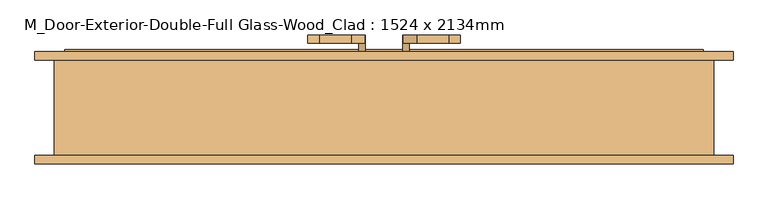
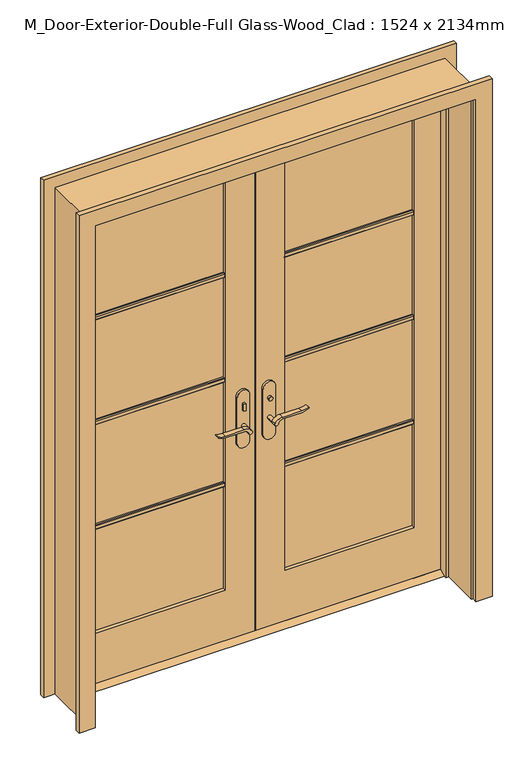
"""IFC4 building model written with IfcOpenShell, lengths in millimetres: door geometry, M_Door-Exterior-Double-Full Glass-Wood_Clad : 1524 x 2134mm."""

from ifc_helpers import new_model, si_unit, point, frame, frame_2d, origin, place, context, project, spatial, polyline, circle_curve, trimmed, segment, composite_curve, outline, extrude, faceted_brep, source, transform, mapped, element, save


def m_door_exterior_double_full_glass_wood_clad_1524_x_2134mm_606f56d5(model_context):
    return source(origin(), model_context, "Body", "SolidModel", [
        extrude(outline(polyline([(76.125, 15.0), (111.125, 15.0), (136.525, 0.0), (50.725, 0.0), (76.125, 15.0)])), frame((-762.0, 0.0, 0.0), z_axis=(1.0, 0.0, 0.0), x_axis=(0.0, 1.0, 0.0)), (0.0, 0.0, 1.0), 1524.0),
        extrude(outline(polyline([(-47.4019111, 56.125), (-57.4019111, 56.125), (-57.4019111, 66.125), (-47.4019111, 66.125), (-47.4019111, 56.125)])), frame((0.0, 0.0, 981.9), z_axis=(0.0, 0.0, 1.0), x_axis=(1.0, 0.0, 0.0)), (0.0, 0.0, 1.0), 30.0),
        extrude(outline(composite_curve([segment(trimmed(circle_curve(frame_2d((996.9, -52.4019111)), 8.0), [point((996.9, -60.4019111))], [point((996.9, -44.4019111))], False, "CARTESIAN"), True, "CONTINUOUS"), segment(trimmed(circle_curve(frame_2d((996.9, -52.4019111)), 8.0), [point((996.9, -44.4019111))], [point((996.9, -60.4019111))], False, "CARTESIAN"), True, "CONTINUOUS")], self_intersect=False)), frame((0.0, 121.125, 0.0), z_axis=(0.0, 1.0, 0.0), x_axis=(0.0, 0.0, 1.0)), (0.0, 0.0, 1.0), 10.0),
        extrude(outline(composite_curve([segment(trimmed(circle_curve(frame_2d((897.1555521, -76.0694241)), 37.2832219), [point((919.0523287, -45.8937749))], [point((934.4, -77.7693445))], False, "CARTESIAN"), True, "CONTINUOUS"), segment(polyline([(934.4, -77.7693445), (934.4, -154.045502)]), True, "CONTINUOUS"), segment(trimmed(circle_curve(frame_2d((1017.6850638, -153.9791202)), 83.2850902), [point((934.4, -154.045502))], [point((939.4, -182.4019111))], True, "CARTESIAN"), True, "CONTINUOUS"), segment(polyline([(939.4, -182.4019111), (936.6135558, -182.4019111)]), True, "CONTINUOUS"), segment(trimmed(circle_curve(frame_2d((986.6709207, -150.4622499)), 59.3791355), [point((936.6135558, -182.4019111))], [point((927.4, -154.045502))], False, "CARTESIAN"), True, "CONTINUOUS"), segment(polyline([(927.4, -154.045502), (927.4, -77.7881013)]), True, "CONTINUOUS"), segment(trimmed(circle_curve(frame_2d((909.2738613, -77.7881013)), 18.1261387), [point((927.4, -77.7881013))], [point((914.4, -60.4019111))], True, "CARTESIAN"), True, "CONTINUOUS"), segment(trimmed(circle_curve(frame_2d((914.4, -52.4019111)), 8.0), [point((914.4, -60.4019111))], [point((919.0523287, -45.8937749))], False, "CARTESIAN"), True, "CONTINUOUS")], self_intersect=False)), frame((0.0, 16.125, 0.0), z_axis=(0.0, 1.0, 0.0), x_axis=(0.0, 0.0, 1.0)), (0.0, 0.0, 1.0), 20.0),
        extrude(outline(composite_curve([segment(trimmed(circle_curve(frame_2d((914.4, -52.4019111)), 8.0), [point((914.3999903, -60.4019111))], [point((919.0523287, -45.8937749))], False, "CARTESIAN"), True, "CONTINUOUS"), segment(trimmed(circle_curve(frame_2d((897.1555521, -76.0694241)), 37.2832219), [point((919.0523287, -45.8937749))], [point((934.4, -77.7693445))], False, "CARTESIAN"), True, "CONTINUOUS"), segment(polyline([(934.4, -77.7693445), (934.4, -154.045502)]), True, "CONTINUOUS"), segment(trimmed(circle_curve(frame_2d((1017.6850638, -153.9791202)), 83.2850902), [point((934.4, -154.045502))], [point((939.4, -182.4019111))], True, "CARTESIAN"), True, "CONTINUOUS"), segment(polyline([(939.4, -182.4019111), (936.6135558, -182.4019111)]), True, "CONTINUOUS"), segment(trimmed(circle_curve(frame_2d((986.6709207, -150.4622499)), 59.3791355), [point((936.6135558, -182.4019111))], [point((927.4, -154.045502))], False, "CARTESIAN"), True, "CONTINUOUS"), segment(polyline([(927.4, -154.045502), (927.4, -77.788099)]), True, "CONTINUOUS"), segment(trimmed(circle_curve(frame_2d((909.2738682, -77.788099)), 18.1261318), [point((927.4, -77.788099))], [point((914.3999903, -60.4019111))], True, "CARTESIAN"), True, "CONTINUOUS")], self_intersect=False)), frame((0.0, 151.125, 0.0), z_axis=(0.0, 1.0, 0.0), x_axis=(0.0, 0.0, 1.0)), (0.0, 0.0, 1.0), 20.0),
        extrude(outline(composite_curve([segment(trimmed(circle_curve(frame_2d((914.4, -52.4019111)), 8.0), [point((914.4, -60.4019111))], [point((914.4, -44.4019111))], False, "CARTESIAN"), True, "CONTINUOUS"), segment(trimmed(circle_curve(frame_2d((914.4, -52.4019111)), 8.0), [point((914.4, -44.4019111))], [point((914.4, -60.4019111))], False, "CARTESIAN"), True, "CONTINUOUS")], self_intersect=False)), frame((0.0, 36.125, 0.0), z_axis=(0.0, 1.0, 0.0), x_axis=(0.0, 0.0, 1.0)), (0.0, 0.0, 1.0), 30.0),
        extrude(outline(composite_curve([segment(trimmed(circle_curve(frame_2d((914.4, -52.4019111)), 8.0), [point((914.4, -60.4019111))], [point((914.4, -44.4019111))], False, "CARTESIAN"), True, "CONTINUOUS"), segment(trimmed(circle_curve(frame_2d((914.4, -52.4019111)), 8.0), [point((914.4, -44.4019111))], [point((914.4, -60.4019111))], False, "CARTESIAN"), True, "CONTINUOUS")], self_intersect=False)), frame((0.0, 121.125, 0.0), z_axis=(0.0, 1.0, 0.0), x_axis=(0.0, 0.0, 1.0)), (0.0, 0.0, 1.0), 30.0),
        extrude(outline(composite_curve([segment(polyline([(844.4, -27.4019111), (1039.4, -27.4019111)]), True, "CONTINUOUS"), segment(trimmed(circle_curve(frame_2d((1039.4, -52.4019111)), 25.0), [point((1039.4, -27.4019111))], [point((1039.4, -77.4019111))], False, "CARTESIAN"), True, "CONTINUOUS"), segment(polyline([(1039.4, -77.4019111), (844.4, -77.4019111)]), True, "CONTINUOUS"), segment(trimmed(circle_curve(frame_2d((844.4, -52.4019111)), 25.0), [point((844.4, -77.4019111))], [point((844.4, -27.4019111))], False, "CARTESIAN"), True, "CONTINUOUS")], self_intersect=False)), frame((0.0, 66.125, 0.0), z_axis=(0.0, 1.0, 0.0), x_axis=(0.0, 0.0, 1.0)), (0.0, 0.0, 1.0), 10.0),
        extrude(outline(composite_curve([segment(polyline([(844.4, -27.4019111), (1039.4, -27.4019111)]), True, "CONTINUOUS"), segment(trimmed(circle_curve(frame_2d((1039.4, -52.4019111)), 25.0), [point((1039.4, -27.4019111))], [point((1039.4, -77.4019111))], False, "CARTESIAN"), True, "CONTINUOUS"), segment(polyline([(1039.4, -77.4019111), (844.4, -77.4019111)]), True, "CONTINUOUS"), segment(trimmed(circle_curve(frame_2d((844.4, -52.4019111)), 25.0), [point((844.4, -77.4019111))], [point((844.4, -27.4019111))], False, "CARTESIAN"), True, "CONTINUOUS")], self_intersect=False)), frame((0.0, 111.125, 0.0), z_axis=(0.0, 1.0, 0.0), x_axis=(0.0, 0.0, 1.0)), (0.0, 0.0, 1.0), 10.0),
        extrude(outline(polyline([(47.3875, 131.125), (57.3875, 131.125), (57.3875, 121.125), (47.3875, 121.125), (47.3875, 131.125)])), frame((0.0, 0.0, 981.9), z_axis=(0.0, 0.0, 1.0), x_axis=(1.0, 0.0, 0.0)), (0.0, 0.0, 1.0), 30.0),
        extrude(outline(composite_curve([segment(trimmed(circle_curve(frame_2d((996.9, 52.3875)), 8.0), [point((996.9, 60.3875))], [point((996.9, 44.3875))], False, "CARTESIAN"), True, "CONTINUOUS"), segment(trimmed(circle_curve(frame_2d((996.9, 52.3875)), 8.0), [point((996.9, 44.3875))], [point((996.9, 60.3875))], False, "CARTESIAN"), True, "CONTINUOUS")], self_intersect=False)), frame((0.0, 56.125, 0.0), z_axis=(0.0, 1.0, 0.0), x_axis=(0.0, 0.0, 1.0)), (0.0, 0.0, 1.0), 10.0),
        extrude(outline(composite_curve([segment(trimmed(circle_curve(frame_2d((914.4, 52.3875)), 8.0), [point((919.0523287, 45.8793637))], [point((914.4, 60.3875))], False, "CARTESIAN"), True, "CONTINUOUS"), segment(trimmed(circle_curve(frame_2d((909.2738613, 77.7736901)), 18.1261387), [point((914.4, 60.3875))], [point((927.4, 77.7736901))], True, "CARTESIAN"), True, "CONTINUOUS"), segment(polyline([(927.4, 77.7736901), (927.4, 154.0310909)]), True, "CONTINUOUS"), segment(trimmed(circle_curve(frame_2d((986.6709207, 150.4478388)), 59.3791355), [point((927.4, 154.0310909))], [point((936.6135558, 182.3875))], False, "CARTESIAN"), True, "CONTINUOUS"), segment(polyline([(936.6135558, 182.3875), (939.4, 182.3875)]), True, "CONTINUOUS"), segment(trimmed(circle_curve(frame_2d((1017.6850638, 153.9647091)), 83.2850902), [point((939.4, 182.3875))], [point((934.4, 154.0310909))], True, "CARTESIAN"), True, "CONTINUOUS"), segment(polyline([(934.4, 154.0310909), (934.4, 77.7549333)]), True, "CONTINUOUS"), segment(trimmed(circle_curve(frame_2d((897.1555521, 76.0550129)), 37.2832219), [point((934.4, 77.7549333))], [point((919.0523287, 45.8793637))], False, "CARTESIAN"), True, "CONTINUOUS")], self_intersect=False)), frame((0.0, 151.125, 0.0), z_axis=(0.0, 1.0, 0.0), x_axis=(0.0, 0.0, 1.0)), (0.0, 0.0, 1.0), 20.0),
        extrude(outline(composite_curve([segment(trimmed(circle_curve(frame_2d((909.2738682, 77.7736878)), 18.1261318), [point((914.3999903, 60.3875))], [point((927.4, 77.7736878))], True, "CARTESIAN"), True, "CONTINUOUS"), segment(polyline([(927.4, 77.7736878), (927.4, 154.0310909)]), True, "CONTINUOUS"), segment(trimmed(circle_curve(frame_2d((986.6709207, 150.4478388)), 59.3791355), [point((927.4, 154.0310909))], [point((936.6135558, 182.3875))], False, "CARTESIAN"), True, "CONTINUOUS"), segment(polyline([(936.6135558, 182.3875), (939.4, 182.3875)]), True, "CONTINUOUS"), segment(trimmed(circle_curve(frame_2d((1017.6850638, 153.9647091)), 83.2850902), [point((939.4, 182.3875))], [point((934.4, 154.0310909))], True, "CARTESIAN"), True, "CONTINUOUS"), segment(polyline([(934.4, 154.0310909), (934.4, 77.7549333)]), True, "CONTINUOUS"), segment(trimmed(circle_curve(frame_2d((897.1555521, 76.0550129)), 37.2832219), [point((934.4, 77.7549333))], [point((919.0523287, 45.8793637))], False, "CARTESIAN"), True, "CONTINUOUS"), segment(trimmed(circle_curve(frame_2d((914.4, 52.3875)), 8.0), [point((919.0523287, 45.8793637))], [point((914.3999903, 60.3875))], False, "CARTESIAN"), True, "CONTINUOUS")], self_intersect=False)), frame((0.0, 16.125, 0.0), z_axis=(0.0, 1.0, 0.0), x_axis=(0.0, 0.0, 1.0)), (0.0, 0.0, 1.0), 20.0),
        extrude(outline(composite_curve([segment(trimmed(circle_curve(frame_2d((914.4, 52.3875)), 8.0), [point((914.4, 60.3875))], [point((914.4, 44.3875))], False, "CARTESIAN"), True, "CONTINUOUS"), segment(trimmed(circle_curve(frame_2d((914.4, 52.3875)), 8.0), [point((914.4, 44.3875))], [point((914.4, 60.3875))], False, "CARTESIAN"), True, "CONTINUOUS")], self_intersect=False)), frame((0.0, 121.125, 0.0), z_axis=(0.0, 1.0, 0.0), x_axis=(0.0, 0.0, 1.0)), (0.0, 0.0, 1.0), 30.0),
        extrude(outline(composite_curve([segment(trimmed(circle_curve(frame_2d((914.4, 52.3875)), 8.0), [point((914.4, 60.3875))], [point((914.4, 44.3875))], False, "CARTESIAN"), True, "CONTINUOUS"), segment(trimmed(circle_curve(frame_2d((914.4, 52.3875)), 8.0), [point((914.4, 44.3875))], [point((914.4, 60.3875))], False, "CARTESIAN"), True, "CONTINUOUS")], self_intersect=False)), frame((0.0, 36.125, 0.0), z_axis=(0.0, 1.0, 0.0), x_axis=(0.0, 0.0, 1.0)), (0.0, 0.0, 1.0), 30.0),
        extrude(outline(composite_curve([segment(trimmed(circle_curve(frame_2d((844.4, 52.3875)), 25.0), [point((844.4, 27.3875))], [point((844.4, 77.3875))], False, "CARTESIAN"), True, "CONTINUOUS"), segment(polyline([(844.4, 77.3875), (1039.4, 77.3875)]), True, "CONTINUOUS"), segment(trimmed(circle_curve(frame_2d((1039.4, 52.3875)), 25.0), [point((1039.4, 77.3875))], [point((1039.4, 27.3875))], False, "CARTESIAN"), True, "CONTINUOUS"), segment(polyline([(1039.4, 27.3875), (844.4, 27.3875)]), True, "CONTINUOUS")], self_intersect=False)), frame((0.0, 111.125, 0.0), z_axis=(0.0, 1.0, 0.0), x_axis=(0.0, 0.0, 1.0)), (0.0, 0.0, 1.0), 10.0),
        extrude(outline(composite_curve([segment(trimmed(circle_curve(frame_2d((844.4, 52.3875)), 25.0), [point((844.4, 27.3875))], [point((844.4, 77.3875))], False, "CARTESIAN"), True, "CONTINUOUS"), segment(polyline([(844.4, 77.3875), (1039.4, 77.3875)]), True, "CONTINUOUS"), segment(trimmed(circle_curve(frame_2d((1039.4, 52.3875)), 25.0), [point((1039.4, 77.3875))], [point((1039.4, 27.3875))], False, "CARTESIAN"), True, "CONTINUOUS"), segment(polyline([(1039.4, 27.3875), (844.4, 27.3875)]), True, "CONTINUOUS")], self_intersect=False)), frame((0.0, 66.125, 0.0), z_axis=(0.0, 1.0, 0.0), x_axis=(0.0, 0.0, 1.0)), (0.0, 0.0, 1.0), 10.0),
        extrude(outline(polyline([(90.125, 1577.225), (90.125, 1558.175), (83.775, 1558.175), (80.6, 1561.35), (80.6, 1574.05), (83.775, 1577.225), (90.125, 1577.225)])), frame((120.0, 0.0, 0.0), z_axis=(1.0, 0.0, 0.0), x_axis=(0.0, 1.0, 0.0)), (0.0, 0.0, 1.0), 522.0),
        extrude(outline(polyline([(90.125, 1131.325), (90.125, 1112.275), (83.775, 1112.275), (80.6, 1115.45), (80.6, 1128.15), (83.775, 1131.325), (90.125, 1131.325)])), frame((120.0, 0.0, 0.0), z_axis=(1.0, 0.0, 0.0), x_axis=(0.0, 1.0, 0.0)), (0.0, 0.0, 1.0), 522.0),
        extrude(outline(polyline([(90.125, 685.425), (90.125, 666.375), (83.775, 666.375), (80.6, 669.55), (80.6, 682.25), (83.775, 685.425), (90.125, 685.425)])), frame((120.0, 0.0, 0.0), z_axis=(1.0, 0.0, 0.0), x_axis=(0.0, 1.0, 0.0)), (0.0, 0.0, 1.0), 522.0),
        extrude(outline(polyline([(97.125, 1577.225), (103.475, 1577.225), (106.65, 1574.05), (106.65, 1561.35), (103.475, 1558.175), (97.125, 1558.175), (97.125, 1577.225)])), frame((-642.0, 0.0, 0.0), z_axis=(1.0, 0.0, 0.0), x_axis=(0.0, 1.0, 0.0)), (0.0, 0.0, 1.0), 522.0),
        extrude(outline(polyline([(97.125, 1131.325), (103.475, 1131.325), (106.65, 1128.15), (106.65, 1115.45), (103.475, 1112.275), (97.125, 1112.275), (97.125, 1131.325)])), frame((-642.0, 0.0, 0.0), z_axis=(1.0, 0.0, 0.0), x_axis=(0.0, 1.0, 0.0)), (0.0, 0.0, 1.0), 522.0),
        extrude(outline(polyline([(97.125, 685.425), (103.475, 685.425), (106.65, 682.25), (106.65, 669.55), (103.475, 666.375), (97.125, 666.375), (97.125, 685.425)])), frame((-642.0, 0.0, 0.0), z_axis=(1.0, 0.0, 0.0), x_axis=(0.0, 1.0, 0.0)), (0.0, 0.0, 1.0), 522.0),
        extrude(outline(polyline([(97.125, 1577.225), (103.475, 1577.225), (106.65, 1574.05), (106.65, 1561.35), (103.475, 1558.175), (97.125, 1558.175), (97.125, 1577.225)])), frame((120.0, 0.0, 0.0), z_axis=(1.0, 0.0, 0.0), x_axis=(0.0, 1.0, 0.0)), (0.0, 0.0, 1.0), 522.0),
        extrude(outline(polyline([(97.125, 1131.325), (103.475, 1131.325), (106.65, 1128.15), (106.65, 1115.45), (103.475, 1112.275), (97.125, 1112.275), (97.125, 1131.325)])), frame((120.0, 0.0, 0.0), z_axis=(1.0, 0.0, 0.0), x_axis=(0.0, 1.0, 0.0)), (0.0, 0.0, 1.0), 522.0),
        extrude(outline(polyline([(97.125, 685.425), (103.475, 685.425), (106.65, 682.25), (106.65, 669.55), (103.475, 666.375), (97.125, 666.375), (97.125, 685.425)])), frame((120.0, 0.0, 0.0), z_axis=(1.0, 0.0, 0.0), x_axis=(0.0, 1.0, 0.0)), (0.0, 0.0, 1.0), 522.0),
        extrude(outline(polyline([(90.125, 1577.225), (90.125, 1558.175), (83.775, 1558.175), (80.6, 1561.35), (80.6, 1574.05), (83.775, 1577.225), (90.125, 1577.225)])), frame((-642.0, 0.0, 0.0), z_axis=(1.0, 0.0, 0.0), x_axis=(0.0, 1.0, 0.0)), (0.0, 0.0, 1.0), 522.0),
        extrude(outline(polyline([(90.125, 1131.325), (90.125, 1112.275), (83.775, 1112.275), (80.6, 1115.45), (80.6, 1128.15), (83.775, 1131.325), (90.125, 1131.325)])), frame((-642.0, 0.0, 0.0), z_axis=(1.0, 0.0, 0.0), x_axis=(0.0, 1.0, 0.0)), (0.0, 0.0, 1.0), 522.0),
        extrude(outline(polyline([(90.125, 685.425), (90.125, 666.375), (83.775, 666.375), (80.6, 669.55), (80.6, 682.25), (83.775, 685.425), (90.125, 685.425)])), frame((-642.0, 0.0, 0.0), z_axis=(1.0, 0.0, 0.0), x_axis=(0.0, 1.0, 0.0)), (0.0, 0.0, 1.0), 522.0),
        extrude(outline(polyline([(0.0, 768.35), (0.0, 833.35), (2204.95, 833.35), (2204.95, -833.35), (0.0, -833.35), (0.0, -768.35), (2139.95, -768.35), (2139.95, 768.35), (0.0, 768.35)])), frame((0.0, 111.125, 0.0), z_axis=(0.0, 1.0, 0.0), x_axis=(0.0, 0.0, 1.0)), (0.0, 0.0, 1.0), 20.0),
        extrude(outline(polyline([(0.0, 768.35), (0.0, 833.35), (2204.95, 833.35), (2204.95, -833.35), (0.0, -833.35), (0.0, -768.35), (2139.95, -768.35), (2139.95, 768.35), (0.0, 768.35)])), frame((0.0, -137.475, 0.0), z_axis=(0.0, 1.0, 0.0), x_axis=(0.0, 0.0, 1.0)), (0.0, 0.0, 1.0), 20.0),
        extrude(outline(polyline([(15.0, 762.0), (2133.6, 762.0), (2133.6, 1.5875), (15.0, 1.5875), (15.0, 762.0)]), holes=[polyline([(2013.6, 120.0), (2013.6, 642.0), (230.0, 642.0), (230.0, 120.0), (2013.6, 120.0)])]), frame((0.0, 76.125, 0.0), z_axis=(0.0, 1.0, 0.0), x_axis=(0.0, 0.0, 1.0)), (0.0, 0.0, 1.0), 35.0),
        extrude(outline(polyline([(2133.6, -762.0), (15.0, -762.0), (15.0, -1.6019111), (2133.6, -1.6019111), (2133.6, -762.0)]), holes=[polyline([(230.0, -642.0), (2013.6, -642.0), (2013.6, -120.0), (230.0, -120.0), (230.0, -642.0)])]), frame((0.0, 76.125, 0.0), z_axis=(0.0, 1.0, 0.0), x_axis=(0.0, 0.0, 1.0)), (0.0, 0.0, 1.0), 35.0),
        faceted_brep([(787.0, 111.125, 0.0), (787.0, -117.475, 0.0), (762.0, -117.475, 0.0), (762.0, 41.2, 0.0), (749.3, 41.2, 0.0), (749.3, 76.125, 0.0), (762.0, 76.125, 0.0), (762.0, 111.125, 0.0), (787.0, 111.125, 2158.6), (787.0, -117.475, 2158.6), (-787.0, -117.475, 2158.6), (-787.0, -117.475, 0.0), (-762.0, -117.475, 0.0), (-762.0, -117.475, 2133.6), (762.0, -117.475, 2133.6), (762.0, 41.2, 2133.6), (-762.0, 41.2, 2133.6), (-762.0, 41.2, 0.0), (-749.3, 41.2, 0.0), (-749.3, 41.2, 2120.9), (749.3, 41.2, 2120.9), (749.3, 76.125, 2120.9), (1.5875, 76.125, 2120.9), (-1.6019111, 76.125, 2120.9), (-749.3, 76.125, 2120.9), (-749.3, 76.125, 0.0), (-762.0, 76.125, 0.0), (-762.0, 76.125, 2133.6), (-1.6019111, 76.125, 2133.6), (1.5875, 76.125, 2133.6), (762.0, 76.125, 2133.6), (762.0, 111.125, 2133.6), (1.5875, 111.125, 2133.6), (-1.6019111, 111.125, 2133.6), (-762.0, 111.125, 2133.6), (-762.0, 111.125, 0.0), (-787.0, 111.125, 0.0), (-787.0, 111.125, 2158.6)], [[[0, 1, 2, 3, 4, 5, 6, 7]], [[1, 0, 8, 9]], [[2, 1, 9, 10, 11, 12, 13, 14]], [[3, 2, 14, 15]], [[4, 3, 15, 16, 17, 18, 19, 20]], [[5, 4, 20, 21]], [[6, 5, 21, 22, 23, 24, 25, 26, 27, 28, 29, 30]], [[7, 6, 30, 31]], [[0, 7, 31, 32, 33, 34, 35, 36, 37, 8]], [[9, 8, 37, 10]], [[14, 13, 16, 15]], [[20, 19, 24, 23, 22, 21]], [[31, 30, 29, 28, 27, 34, 33, 32]], [[12, 11, 36, 35, 26, 25, 18, 17]], [[11, 10, 37, 36]], [[13, 12, 17, 16]], [[19, 18, 25, 24]], [[27, 26, 35, 34]]]),
        extrude(outline(polyline([(642.0, 90.125), (120.0, 90.125), (120.0, 97.125), (642.0, 97.125), (642.0, 90.125)])), frame((0.0, 0.0, 230.0), z_axis=(0.0, 0.0, 1.0), x_axis=(1.0, 0.0, 0.0)), (0.0, 0.0, 1.0), 1783.6),
        extrude(outline(polyline([(-120.0, 90.125), (-642.0, 90.125), (-642.0, 97.125), (-120.0, 97.125), (-120.0, 90.125)])), frame((0.0, 0.0, 230.0), z_axis=(0.0, 0.0, 1.0), x_axis=(1.0, 0.0, 0.0)), (0.0, 0.0, 1.0), 1783.6),
    ])


if __name__ == "__main__":
    model = new_model("IFC4")
    model_context = context("Model", 3, world=origin())
    ifc_project = project(units=[si_unit("LENGTHUNIT", "METRE", prefix="MILLI")], contexts=[model_context])
    site = spatial("IfcSite", under=ifc_project)
    building = spatial("IfcBuilding", under=site)
    placement = place(None, origin())
    m_door_exterior_double_full_glass_wood_clad_1524_x_2134mm_shape = m_door_exterior_double_full_glass_wood_clad_1524_x_2134mm_606f56d5(model_context)
    element("IfcDoor", 1, ObjectType="M_Door-Exterior-Double-Full Glass-Wood_Clad : 1524 x 2134mm", at=placement, inside=building, context=model_context, shape_type="MappedRepresentation", body=[
        mapped(m_door_exterior_double_full_glass_wood_clad_1524_x_2134mm_shape, transform((0.0, 0.0, 0.0), x_axis=(1.0, 0.0, 0.0), y_axis=(0.0, 1.0, 0.0), z_axis=(0.0, 0.0, 1.0))),
    ])
    save(model, "model.ifc")

# Revit data of these elements
# Type "M_Door-Exterior-Double-Full Glass-Wood_Clad : 1524 x 2134mm"
#   Type Mark = "9"
#   Assembly Code = "B2030100"
#   Analytic Construction = "French door, wood frame with double glass"
#   Top Rail = 0' - 4.72441"
#   Threshold Offset [instance default] = 0' - 0.59055"
#   Thickness = 0' - 1.37795"
#   Thermal Resistance (R) = 1.9158 (h·ft²·°F)/BTU
#   Swing Angle [instance default] = 90.00°
#   Stiles = 0' - 4.72441"
#   Rough Width = 5' - 1.9685"
#   Rough Height = 7' - 0.98425"
#   Panel Width = 2' - 6"
#   Door Offset [instance default] = 0' - 0"
#   Height = 7' - 0"
#   Width = 5' - 0"
#   Heat Transfer Coefficient (U) = 0.5220 BTU/(h·ft²·°F)
#   Bottom Rail = 0' - 9.05512"
#   Exterior Trim [instance default] = yes
#   Threshold [instance default] = yes
#   Show Grill [instance default] = yes
#   Function = 1
#   Trim Material = Cherry
#   Threshold Material = Cherry
#   Panel Material = Cherry
#   Glazing = Glass
#   Frame Material = Cherry
#   Door Handle Material = Aluminum
#   Visual Light Transmittance = 0
#   Solar Heat Gain Coefficient = 0
#   Wall Closure = (empty or 0)
#   Construction Type = (empty or 0)
# Element 1 (IfcDoor, "M_Door-Exterior-Double-Full Glass-Wood_Clad : 1524 x 2134mm")
#   Materials on its faces: "Cherry", "Aluminum", "Glass"
# Materials
#   "Cherry": class "Wood", colour RGB 226 177 128, transparency 0, Description = "Prunus Serotina", Cost = 0
#   "Glass": class "Glass", colour RGB 0 128 192, transparency 0.75, Description = "Soda Lime Glass", Cost = 0
#   "Aluminum": class "Metal", colour RGB 247 247 247, transparency 0, Description = "Aluminum 6061", Cost = 0
